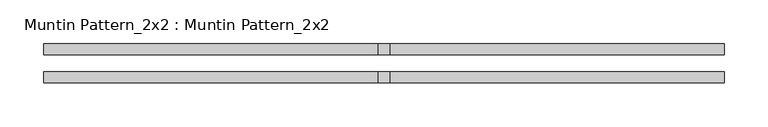
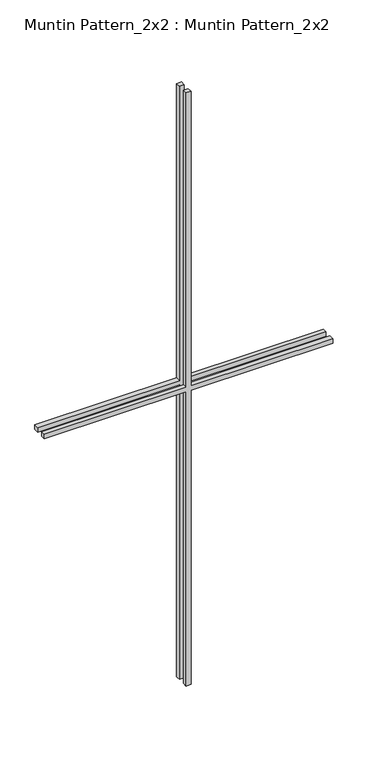
"""IFC4 building model written with IfcOpenShell, lengths in millimetres: proxy geometry, Muntin Pattern_2x2 : Muntin Pattern_2x2."""

from ifc_helpers import new_model, si_unit, frame, origin, place, context, project, spatial, polyline, outline, extrude, source, transform, mapped, element, save


def muntin_pattern_2x2_muntin_pattern_2x2_e6f69628(model_context):
    return source(origin(), model_context, "Body", "SweptSolid", [
        extrude(outline(polyline([(850.9, -6.35), (850.9, -388.9375), (838.2, -388.9375), (838.2, -6.35), (0.0, -6.35), (0.0, 6.35), (838.2, 6.35), (838.2, 388.9375), (850.9, 388.9375), (850.9, 6.35), (1689.1, 6.35), (1689.1, -6.35), (850.9, -6.35)])), frame((0.0, -22.225, 0.0), z_axis=(0.0, 1.0, 0.0), x_axis=(0.0, 0.0, 1.0)), (0.0, 0.0, 1.0), 12.7),
        extrude(outline(polyline([(850.9, -6.35), (850.9, -388.9375), (838.2, -388.9375), (838.2, -6.35), (0.0, -6.35), (0.0, 6.35), (838.2, 6.35), (838.2, 388.9375), (850.9, 388.9375), (850.9, 6.35), (1689.1, 6.35), (1689.1, -6.35), (850.9, -6.35)])), frame((0.0, 9.525, 0.0), z_axis=(0.0, 1.0, 0.0), x_axis=(0.0, 0.0, 1.0)), (0.0, 0.0, 1.0), 12.7),
    ])


if __name__ == "__main__":
    model = new_model("IFC4")
    model_context = context("Model", 3, world=origin())
    ifc_project = project(units=[si_unit("LENGTHUNIT", "METRE", prefix="MILLI")], contexts=[model_context])
    site = spatial("IfcSite", under=ifc_project)
    building = spatial("IfcBuilding", under=site)
    placement = place(None, origin())
    muntin_pattern_2x2_muntin_pattern_2x2_shape = muntin_pattern_2x2_muntin_pattern_2x2_e6f69628(model_context)
    element("IfcBuildingElementProxy", 1, Name="Muntin Pattern_2x2 : Muntin Pattern_2x2", ObjectType="Muntin Pattern_2x2 : Muntin Pattern_2x2", at=placement, inside=building, context=model_context, shape_type="MappedRepresentation", body=[
        mapped(muntin_pattern_2x2_muntin_pattern_2x2_shape, transform((0.0, 0.0, 0.0), x_axis=(1.0, 0.0, 0.0), y_axis=(0.0, 1.0, 0.0), z_axis=(0.0, 0.0, 1.0))),
    ])
    save(model, "model.ifc")

# Revit data of these elements
# Type "Muntin Pattern_2x2 : Muntin Pattern_2x2"
#   Width [instance default] = 4' - 0"
#   Thickness = 0' - 0 1/2"
#   Height [instance default] = 4' - 0"
#   Distance = 0' - 0 3/4"
#   Interior Material [instance default] = none
#   Exterior Material [instance default] = none
#   Default Elevation = 0
# Element 1 (IfcBuildingElementProxy, "Muntin Pattern_2x2 : Muntin Pattern_2x2")
#   Width = 2' - 6 5/8"
#   Height = 5' - 6 1/2"
#   Interior Material = Wood - Stained
#   Exterior Material = Clad - White
#   Materials on its faces: "Clad - White", "Wood - Stained"
# Materials
#   "Clad - White": class "Wood", colour RGB 242 242 238, transparency 0, Cost = 0
#   "Wood - Stained": class "Wood", colour RGB 224 178 126, transparency 0, Cost = 0
